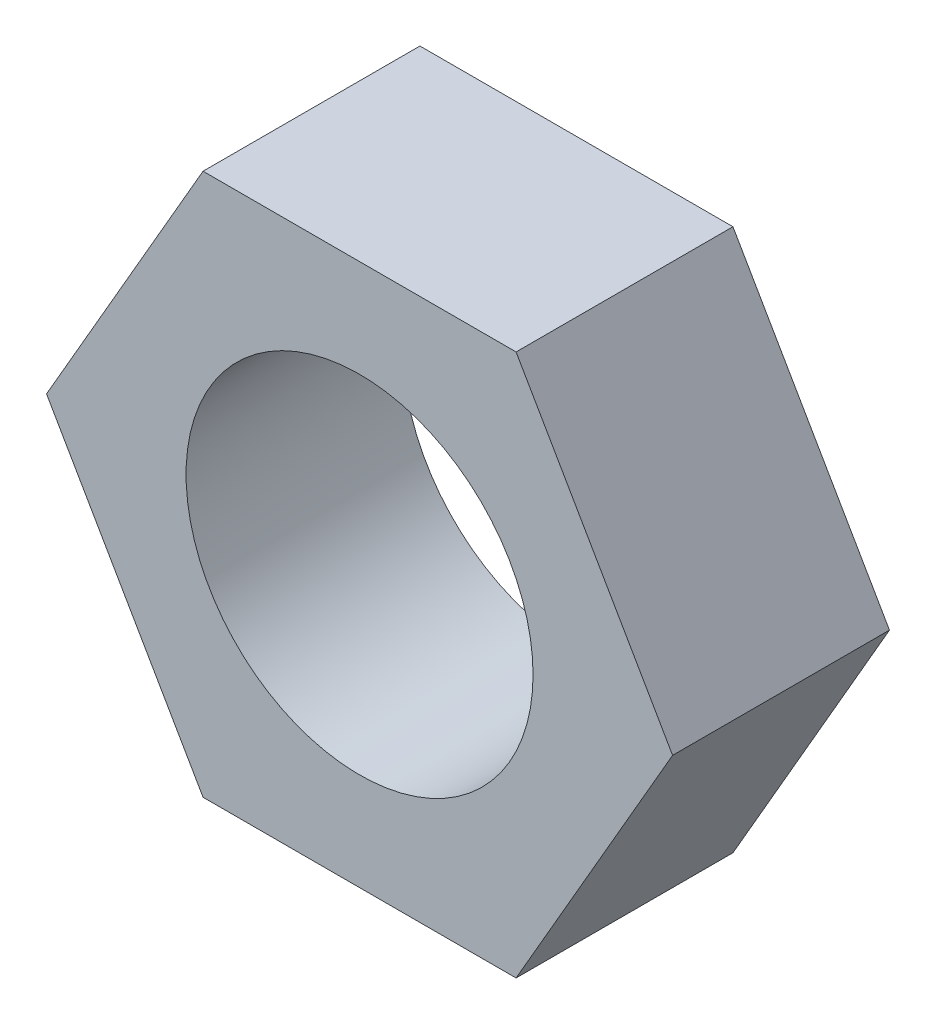
SolidWorks part; units mm, degrees
material "Plain Carbon Steel"
ref_plane "Front Plane" through (0, 0, 0) normal (0, 0, 1) x (1, 0, 0)
ref_plane "Top Plane" through (0, 0, 0) normal (0, 1, 0) x (1, 0, 0)
ref_plane "Right Plane" through (0, 0, 0) normal (1, 0, 0) x (0, 0, -1)
sketch "Hex Profile Sketch 25AF" plane through (0, 0, 0) normal (0, 0, 1) x (1, 0, 0)
  line L0 (0, 25.1147) -> (0, -22.228) construction
  line L1 (38.4259, 0) -> (-35.6674, 0) construction
  line L3 (14.4338, 0) -> (7.2169, 12.5)
  line L4 (7.2169, 12.5) -> (-7.2169, 12.5)
  line L5 (-7.2169, 12.5) -> (-14.4338, 0)
  line L6 (-14.4338, 0) -> (-7.2169, -12.5)
  line L7 (-7.2169, -12.5) -> (7.2169, -12.5)
  line L8 (7.2169, -12.5) -> (14.4338, 0)
  circle A0 centre (0, 0) radius 12.5 construction
  dimension "D1" = 25
extrude "Hex Body 25AF x10" add sketch "Hex Profile Sketch 25AF" along normal blind 10
sketch "Bore Sketch Ø16" plane through (0, 0, 10) normal (0, 0, 1) x (1, 0, 0)
  circle A0 centre (0, 0) radius 8
  dimension "D1" = 16
extrude "Bore Ø16" cut sketch "Bore Sketch Ø16" against normal blind 10
